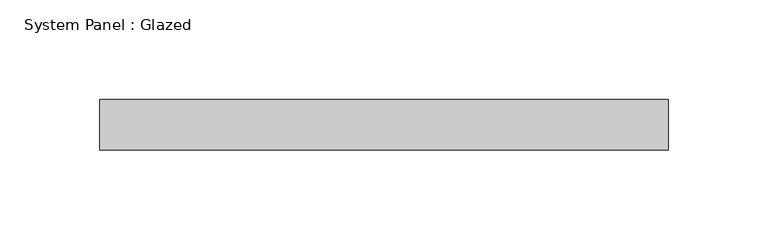
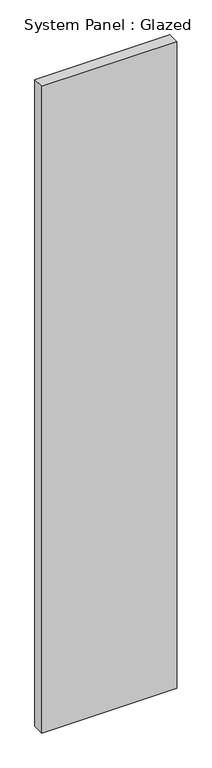
"""IFC4 building model written with IfcOpenShell, lengths in millimetres: plate geometry, System Panel : Glazed."""

from ifc_helpers import new_model, si_unit, origin, origin_with_axes, place, context, project, spatial, polyline, outline, extrude, source, transform, mapped, element, save


def system_panel_glazed_c33e710a(model_context):
    return source(origin(), model_context, "Body", "SweptSolid", [
        extrude(outline(polyline([(142.875, 19.05), (-142.875, 19.05), (-142.875, 44.45), (142.875, 44.45), (142.875, 19.05)])), origin_with_axes(), (0.0, 0.0, 1.0), 1447.2288132),
    ])


if __name__ == "__main__":
    model = new_model("IFC4")
    model_context = context("Model", 3, world=origin())
    ifc_project = project(units=[si_unit("LENGTHUNIT", "METRE", prefix="MILLI")], contexts=[model_context])
    site = spatial("IfcSite", under=ifc_project)
    building = spatial("IfcBuilding", under=site)
    placement = place(None, origin())
    system_panel_glazed_shape = system_panel_glazed_c33e710a(model_context)
    element("IfcPlate", 1, ObjectType="System Panel : Glazed", at=placement, inside=building, context=model_context, shape_type="MappedRepresentation", body=[
        mapped(system_panel_glazed_shape, transform((0.0, 0.0, 0.0), x_axis=(1.0, 0.0, 0.0), y_axis=(0.0, 1.0, 0.0), z_axis=(0.0, 0.0, 1.0))),
    ])
    save(model, "model.ifc")

# Revit data of these elements
# Type "System Panel : Glazed"
#   Construction Type Id = "GSP4R"
#   Analytic Construction = "1/8 in Pilkington single glazing"
#   Visual Light Transmittance = 0.9
#   Solar Heat Gain Coefficient = 0.86
#   Heat Transfer Coefficient (U) = 1.18115 BTU/(h·ft²·°F)
#   Define Thermal Properties by = 1
# Element 1 (IfcPlate, "System Panel : Glazed")
#   Materials on its faces: "Glass"
# Materials
#   "Glass": class "Glass", colour RGB 0 128 192, transparency 0.75, Description = "Soda Lime Glass", Cost = 0
